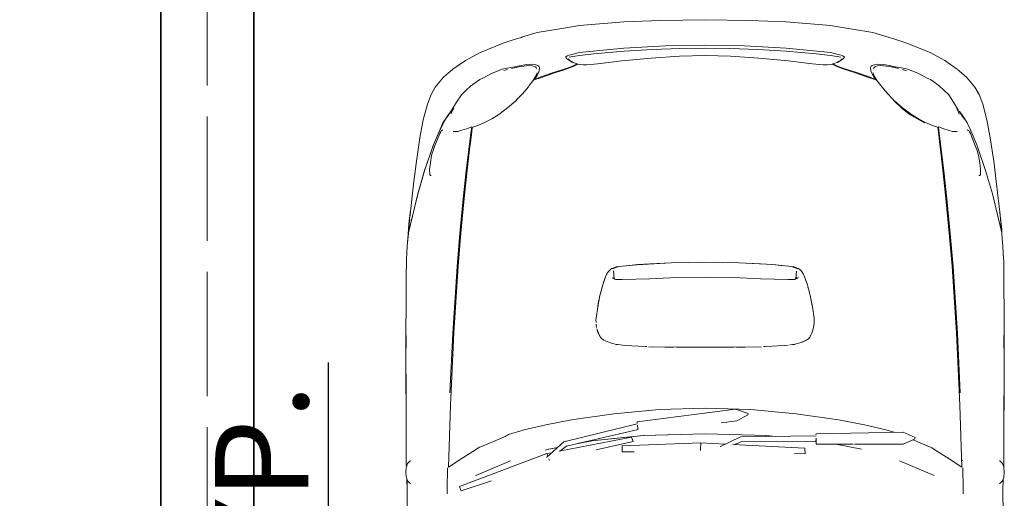
# Model space of a CAD drawing. Units: millimetres. Extents: x 595116 to 630915, y 909473 to 920225.
# Tile 117 of 134: x 629298 to 629393, y 919512 to 919558. Entities that reach past the tile are written whole.
import ezdxf

# ---------------------------------------------------------------- set-up
doc = ezdxf.new("R2010")
doc.units = ezdxf.units.MM
doc.linetypes.add('ACAD_ISO02W100', pattern=[15, 12, -3])
for name, color, linetype, lineweight in [('A-WALL', 1, 'Continuous', 35), ('C-PRKG-VEHI', 8, 'Continuous', 13), ('C-PROP-REF', 240, 'ACAD_ISO02W100', 13), ('Dimension', 3, 'Continuous', 18)]:
    doc.layers.add(name, color=color, linetype=linetype, lineweight=lineweight)
doc.styles.get("Standard").update_dxf_attribs({"font": 'arial.ttf'})
doc.dimstyles.new('ISO-25', dxfattribs={"dimtxt": 9, "dimasz": 6, "dimexe": 1.25, "dimexo": 0.625, "dimtad": 1, "dimlunit": 4, "dimtxsty": 'Standard', "dimcen": 2.5, "dimadec": 0, "dimazin": 0, "dimtfac": 1, "dimtmove": 0, "dimatfit": 3, "dimfxl": 1, "dimarcsym": 0})

# ---------------------------------------------------------------- blocks, each defined once
blk = doc.blocks.new('A$C7ADB3080')
for p, q in [((574.5, 1827.8), (485.6, 1817.6)), ((514, 1805.8), (622.7, 1832)), ((568.1, 1827.1), (601.7, 1831.6)), ((596.5, 1830), (587.6, 1828.8)), ((596.5, 1830), (598.5, 1830.3)), ((598.5, 1830.3), (629.8, 1833.4)), ((615.8, 1832.9), (601.7, 1831.6)), ((629.8, 1833.4), (615.8, 1832.9)), ((622.7, 1832), (625.4, 1832.6)), ((625.4, 1832.6), (622.7, 1832)), ((625.4, 1832.6), (627.4, 1832.8)), ((627.4, 1832.8), (625.4, 1832.6)), ((627.4, 1832.8), (629.3, 1833)), ((629.3, 1833), (627.4, 1832.8)), ((630.2, 1833.1), (628.2, 1832.8)), ((644.6, 1834.3), (629.8, 1833.4)), ((666, 1836.1), (630.2, 1833.1)), ((702.2, 1838.3), (666, 1836.1)), ((702.2, 1838.3), (704.4, 1838.4)), ((755.9, 1839.2), (704.4, 1838.4)), ((755.9, 1839.2), (789.1, 1839)), ((846.4, 1839.7), (789.1, 1839)), ((900.9, 1840.1), (846.4, 1839.7)), ((947, 1840.2), (900.9, 1840.1)), ((998.4, 1839.9), (923, 1839.2)), ((1014.5, 1840), (947, 1840.2)), ((998.4, 1839.9), (1014.5, 1840)), ((1066.5, 1839.8), (1014.5, 1840)), ((1117.5, 1839.5), (1066.5, 1839.8)), ((1120.4, 1839.3), (1070.3, 1839.6)), ((1164.2, 1839.3), (1117.5, 1839.5)), ((1120.4, 1839.3), (1164.2, 1839.1)), ((1164.2, 1839.1), (1164.1, 1839.1)), ((1186, 1839.2), (1164.2, 1839.3)), ((1211.9, 1839.1), (1164.4, 1839.2)), ((1256.2, 1839), (1211.9, 1839.1)), ((1295.5, 1839), (1256.2, 1839)), ((1284.8, 1825.7), (1285.6, 1828.2)), ((1285.6, 1828.2), (1292.6, 1835.1)), ((1292.6, 1835.1), (1302.3, 1838.5)), ((1295.5, 1839), (1302.9, 1838.7)), ((1302.3, 1838.5), (1304.4, 1839)), ((1304.4, 1839), (1317.7, 1840)), ((1331.1, 1839.1), (1317.7, 1840)), ((1331.1, 1839.1), (1333.2, 1838.5)), ((1342.9, 1835.1), (1333.2, 1838.5)), ((1336.7, 1837.3), (1371.1, 1836.1)), ((1349.8, 1828.2), (1342.9, 1835.1)), ((1350.6, 1825.4), (1349.8, 1828.2)), ((1371.1, 1836.1), (1377.3, 1836)), ((1377.3, 1836), (1430.5, 1836.5)), ((352.3, 1799.8), (300.5, 1789.8)), ((419.3, 1809.7), (352.3, 1799.8)), ((485.6, 1817.6), (419.3, 1809.7)), ((446.6, 1786.3), (514, 1805.8)), ((514, 1805.8), (446.6, 1786.3)), ((227, 1767.4), (205.8, 1755.4)), ((255.3, 1777.9), (227, 1767.4)), ((300.5, 1789.8), (255.3, 1777.9)), ((372.4, 1760.5), (446.6, 1786.3)), ((446.6, 1786.3), (372.4, 1760.5)), ((396.8, 1764.1), (391.9, 1762.5)), ((403.1, 1765.7), (396.8, 1764.1)), ((424.7, 1769.2), (403.1, 1765.7)), ((443.9, 1771.4), (424.7, 1769.2)), ((457.6, 1771.3), (443.9, 1771.4)), ((461, 1769.1), (457.6, 1771.3)), ((461.4, 1766.7), (461, 1769.1)), ((205.8, 1755.4), (177.4, 1731.2)), ((308.8, 1733), (327.4, 1741.3)), ((327.4, 1741.3), (308.8, 1733)), ((327.4, 1741.3), (372.4, 1760.5)), ((372.4, 1760.5), (327.4, 1741.3)), ((329.5, 1733), (330.6, 1736)), ((331.4, 1737.3), (330.6, 1736)), ((334.6, 1739.6), (331.4, 1737.3)), ((339.6, 1742.2), (334.6, 1739.6)), ((377.1, 1757.2), (339.6, 1742.2)), ((385.9, 1760.4), (377.1, 1757.2)), ((391.9, 1762.5), (385.9, 1760.4)), ((177.4, 1731.2), (154.5, 1704.8)), ((248.7, 1693.9), (272.8, 1708.2)), ((272.8, 1708.2), (248.7, 1693.9)), ((274.1, 1706.2), (268.7, 1703.4)), ((278, 1711.4), (275.4, 1709.5)), ((275.5, 1706.9), (283.4, 1709.5)), ((276.7, 1711.4), (284.8, 1717.1)), ((287.5, 1718), (278, 1711.4)), ((284.8, 1717.1), (296.4, 1724.9)), ((298.6, 1725.5), (287.5, 1718)), ((296.4, 1724.9), (308.8, 1733)), ((308.8, 1733), (296.4, 1724.9)), ((1124.1, 1711.4), (915.2, 1701.7)), ((917.2, 1704.7), (1089.1, 1712.9)), ((1303.7, 1717.2), (1124.1, 1711.4)), ((1279.1, 1680.6), (1303.7, 1717.2)), ((1284, 1719.6), (1282.1, 1716.5)), ((1304.9, 1720.3), (1365.2, 1721)), ((1365.2, 1721), (1380.7, 1721.1)), ((128.8, 1668.1), (153.9, 1704.5)), ((214.1, 1665.8), (228.3, 1679.7)), ((228.3, 1679.7), (214.1, 1665.8)), ((228.3, 1679.7), (248.7, 1693.9)), ((248.7, 1693.9), (228.3, 1679.7)), ((330.2, 1678.1), (326.2, 1665.2)), ((333.4, 1690.2), (330.2, 1678.1)), ((333.6, 1703.6), (333.4, 1690.2)), ((627.3, 1681.1), (536.8, 1672.6)), ((538.3, 1675.5), (628.6, 1684.1)), ((722.4, 1689.2), (627.3, 1681.1)), ((628.6, 1684.1), (723.6, 1692.3)), ((915.2, 1701.7), (722.4, 1689.2)), ((723.6, 1692.3), (917.2, 1704.7)), ((1257.7, 1647.2), (1279.1, 1680.6)), ((106.5, 1627.7), (128.8, 1668.1)), ((192.9, 1640.1), (202.7, 1653)), ((202.7, 1653), (192.9, 1640.1)), ((202.7, 1653), (214.1, 1665.8)), ((214.1, 1665.8), (202.7, 1653)), ((316.4, 1632.4), (321.9, 1649.9)), ((326.2, 1665.2), (320.7, 1650)), ((320.7, 1650), (340.1, 1652.4)), ((320.7, 1649.8), (320.7, 1650)), ((320.7, 1650), (321, 1650)), ((343.5, 1650.7), (321.3, 1648)), ((321.9, 1649.9), (322, 1650.2)), ((340.1, 1652.4), (392.9, 1659.3)), ((371.1, 1654.1), (343.5, 1650.7)), ((401.8, 1657.9), (371.1, 1654.1)), ((392.9, 1659.3), (455.7, 1666.7)), ((454.1, 1664), (401.8, 1657.9)), ((536.8, 1672.6), (454.1, 1664)), ((455.7, 1666.7), (538.2, 1675.4)), ((538.2, 1675.4), (538.2, 1675.4)), ((538.3, 1675.5), (538.3, 1675.5)), ((78.4, 1559.2), (106.5, 1627.7)), ((179.4, 1617.7), (183.6, 1626.9)), ((183.6, 1626.9), (179.4, 1617.7)), ((183.6, 1626.9), (192.9, 1640.1)), ((192.9, 1640.1), (183.6, 1626.9)), ((308, 1612.7), (316.4, 1632.4)), ((1224.6, 1577), (1244.4, 1624.1)), ((1244.4, 1624.1), (1245.8, 1627.5)), ((1245.8, 1627.5), (1247.6, 1630.5)), ((1247.6, 1630.5), (1257.7, 1647.2)), ((1285.5, 1538), (1327.9, 1638.1)), ((154.1, 1561.6), (166.6, 1592.6)), ((166.6, 1592.6), (154.1, 1561.6)), ((166.6, 1592.6), (179.4, 1617.7)), ((179.4, 1617.7), (166.6, 1592.6)), ((284.8, 1567.7), (299.6, 1592.1)), ((285.2, 1572), (297.6, 1592.1)), ((297.6, 1592.1), (308, 1612.7)), ((299.6, 1592.1), (308.6, 1609.9)), ((265.7, 1546.2), (285.2, 1572)), ((284.8, 1567.7), (268.5, 1546.6)), ((284.8, 1567.7), (284.7, 1567.6)), ((1201.9, 1547.7), (1217.9, 1583.1)), ((1223, 1580.9), (1217.9, 1583.1)), ((1236.7, 1548.1), (1223, 1580.9)), ((70.3, 1532.9), (78.4, 1559.2)), ((147.2, 1525.2), (150.6, 1548.3)), ((150.6, 1548.3), (147.2, 1525.2)), ((150.6, 1548.3), (154.1, 1561.6)), ((154.1, 1561.6), (150.6, 1548.3)), ((158.2, 1557.5), (154.9, 1546.4)), ((245.7, 1523), (265.7, 1546.2)), ((268.5, 1546.6), (247.9, 1525.1)), ((1207.6, 1296.6), (1201.9, 1547.7)), ((1236.9, 1407.5), (1236.7, 1548.1)), ((1285.3, 1537.6), (1285.5, 1538)), ((62.1, 1506.7), (66.6, 1521)), ((66.6, 1521), (70.3, 1532.9)), ((140.7, 1492.2), (144.6, 1512.1)), ((144.6, 1512.1), (140.7, 1492.2)), ((145.9, 1508), (143.4, 1483.5)), ((144.6, 1512.1), (147.2, 1525.2)), ((147.2, 1525.2), (144.6, 1512.1)), ((150.3, 1526.6), (145.9, 1508)), ((152.2, 1535), (150.3, 1526.6)), ((237.6, 1515.3), (225.8, 1504.4)), ((247.9, 1525.1), (237.6, 1515.3)), ((1195.1, 1498.2), (1202.5, 1522)), ((61.6, 1504.8), (48.4, 1460.7)), ((61.6, 1504.8), (62.1, 1506.7)), ((139.4, 1475.5), (140.7, 1492.2)), ((140.7, 1492.2), (139.4, 1475.5)), ((143.4, 1483.5), (144.5, 1474.1)), ((201, 1483.7), (187.2, 1473)), ((204.5, 1486.1), (201, 1483.7)), ((217.4, 1496.7), (204.5, 1486.1)), ((225.8, 1504.4), (217.4, 1496.7)), ((1180.7, 1436.4), (1195.1, 1498.2)), ((48.4, 1460.7), (38.4, 1401.7)), ((140.1, 1468.1), (139.4, 1475.5)), ((139.4, 1475.5), (140.1, 1468.1)), ((143.2, 1458.9), (140.1, 1468.1)), ((140.1, 1468.1), (143.2, 1458.9)), ((145, 1456.1), (143.2, 1458.9)), ((143.2, 1458.9), (145, 1456.1)), ((144.5, 1474.1), (146.2, 1469.1)), ((148.9, 1454.2), (145, 1456.1)), ((145, 1456.1), (148.9, 1454.2)), ((146.5, 1468.2), (149.1, 1464)), ((160, 1454.9), (148.9, 1454.2)), ((148.9, 1454.2), (160, 1454.9)), ((149.1, 1464), (151.7, 1462.6)), ((172.4, 1461.2), (160, 1454.9)), ((160, 1454.9), (172.4, 1461.2)), ((162.7, 1410.7), (176.1, 1450.1)), ((164.5, 1461.2), (172.2, 1463.8)), ((178.9, 1450.6), (164.5, 1410.7)), ((172, 1462.5), (184.5, 1470.4)), ((172.2, 1463.8), (181.7, 1469.2)), ((183.7, 1468.4), (172.4, 1461.2)), ((172.4, 1461.2), (183.7, 1468.4)), ((174.2, 1464.8), (173.9, 1464.7)), ((174.8, 1465.1), (174.2, 1464.8)), ((176.1, 1450.1), (183.7, 1468.4)), ((184.7, 1470.2), (178.9, 1450.6)), ((181.7, 1469.2), (186.7, 1472.5)), ((183.5, 1468), (184.1, 1468.1)), ((183.7, 1468.4), (184.5, 1470.4)), ((184, 1469.2), (184.5, 1469.5)), ((184.1, 1469.5), (184.6, 1469.7)), ((184.5, 1470.4), (185.1, 1470.6)), ((187.2, 1473), (184.7, 1470.2)), ((1166.8, 1361.5), (1180.7, 1436.4)), ((1237, 1353.9), (1251.4, 1427.7)), ((27.8, 1338.5), (38.4, 1401.7)), ((154.5, 1385.6), (162.7, 1410.7)), ((164.5, 1410.7), (156.5, 1386)), ((1237.1, 1297.2), (1236.9, 1403.7)), ((112.3, 1364.4), (113.8, 1369.4)), ((113.8, 1369.4), (112.3, 1364.4)), ((113.8, 1369.4), (115.5, 1374.4)), ((115.5, 1374.4), (113.8, 1369.4)), ((115.5, 1374.4), (118, 1378)), ((118, 1378), (115.5, 1374.4)), ((118.7, 1368.1), (117, 1357.9)), ((118, 1378), (119.5, 1378.4)), ((119.5, 1378.4), (118, 1378)), ((119.5, 1378.4), (123.8, 1375.2)), ((123.8, 1375.2), (119.5, 1378.4)), ((123.7, 1371.6), (127.9, 1368.1)), ((123.8, 1375.2), (127.7, 1369.2)), ((127.7, 1369.2), (123.8, 1375.2)), ((127.7, 1369.2), (133.5, 1360.1)), ((133.5, 1360.1), (127.7, 1369.2)), ((127.9, 1368.1), (131.7, 1361.7)), ((145.3, 1358.5), (150.2, 1371.5)), ((151.3, 1369.4), (145.6, 1354.8)), ((150.2, 1371.5), (154.5, 1385.6)), ((156.5, 1386), (151.3, 1369.4)), ((27.8, 1338.5), (17, 1210.7)), ((93.5, 1210.7), (105.3, 1338.7)), ((105.3, 1338.7), (93.5, 1210.7)), ((105.3, 1338.7), (112.3, 1364.4)), ((112.3, 1364.4), (105.3, 1338.7)), ((114.6, 1338.6), (109.6, 1297.4)), ((117, 1357.9), (114.6, 1338.6)), ((131.7, 1361.7), (134.5, 1357.5)), ((133.5, 1360.1), (137.9, 1348.2)), ((137.9, 1348.2), (133.5, 1360.1)), ((137.9, 1348.2), (138.7, 1345.5)), ((138.7, 1345.5), (137.9, 1348.2)), ((138.7, 1345.5), (145.3, 1358.5)), ((140.3, 1345.5), (138.7, 1345.5)), ((145.6, 1354.8), (139.2, 1343.6)), ((139.2, 1343.6), (140.6, 1338.5)), ((140.1, 1345.5), (140.2, 1345.3)), ((140.6, 1338.5), (141.3, 1328.4)), ((1149.4, 1239.2), (1166.8, 1361.5)), ((141, 1317.4), (140.1, 1305.8)), ((141.3, 1328.4), (141, 1317.4)), ((109.6, 1297.4), (102.1, 1210)), ((138.4, 1286.6), (135.7, 1262.5)), ((140.1, 1305.8), (138.4, 1286.6)), ((807.2, 1279.5), (776.6, 1271.5)), ((840.1, 1286.2), (807.2, 1279.5)), ((816.8, 1281.5), (831.5, 1284.8)), ((831.5, 1284.8), (838.3, 1285.8)), ((873.1, 1290.9), (840.1, 1286.2)), ((888.8, 1291.1), (873.1, 1290.9)), ((873.2, 1290.9), (876.6, 1291.3)), ((876.6, 1291.3), (884.9, 1291)), ((903.4, 1288.7), (888.8, 1291.1)), ((890.4, 1290.8), (894.1, 1290.7)), ((894.1, 1290.7), (899.9, 1289.3)), ((916.5, 1284.3), (903.4, 1288.7)), ((906.8, 1287.6), (908, 1287.3)), ((908, 1287.3), (916.4, 1284.4)), ((916.4, 1284.4), (923.9, 1280.5)), ((927.7, 1278.5), (916.5, 1284.3)), ((923.9, 1280.5), (924.7, 1280.1)), ((1207.6, 1296.6), (1209.6, 1296.4)), ((1215.8, 1078.8), (1213.2, 1296.7)), ((1227.6, 1296), (1219.5, 1296.9)), ((1222.6, 1296.6), (1237.1, 1297.2)), ((1226.3, 1296.1), (1226.4, 1296.8)), ((1230.4, 1295.7), (1227.6, 1296)), ((1229.7, 1083), (1230.4, 1295.7)), ((135.7, 1262.5), (129.8, 1216.2)), ((737.5, 1254.5), (732.6, 1249.6)), ((743.3, 1258.9), (737.5, 1254.5)), ((750.3, 1262.4), (743.3, 1258.9)), ((744.9, 1259.7), (745.5, 1260.1)), ((745.5, 1260.1), (746.8, 1260.6)), ((776.6, 1271.5), (750.3, 1262.4)), ((755.5, 1264.2), (760.9, 1266.4)), ((760.9, 1266.4), (769.9, 1269.2)), ((783.2, 1273.2), (791.1, 1275.6)), ((791.1, 1275.6), (800.2, 1277.7)), ((931.6, 1275.4), (927.7, 1278.5)), ((928.5, 1277.9), (929.6, 1277.2)), ((929.6, 1277.2), (930.1, 1276.6)), ((934.3, 1272), (931.6, 1275.4)), ((936.3, 1268.2), (934.3, 1272)), ((935.3, 1270), (936.3, 1268.7)), ((936.3, 1268.7), (941.9, 1256.9)), ((938.5, 1264), (936.3, 1268.2)), ((944.5, 1249.5), (938.5, 1264)), ((941.9, 1256.9), (943, 1253.2)), ((1248.6, 1264.5), (1238.1, 1056.7)), ((1264.7, 1265), (1248.6, 1264.5)), ((1263.8, 1234.3), (1264.7, 1265)), ((724, 1225.9), (718.5, 1171.5)), ((730.7, 1243.7), (724, 1225.9)), ((724.5, 1227.4), (725.2, 1233.3)), ((725.2, 1233.3), (729.7, 1243.8)), ((732.6, 1249.6), (728.6, 1244.4)), ((728.6, 1244.4), (730.5, 1243.3)), ((733.1, 1250.3), (733, 1250.1)), ((733.3, 1250.3), (733.1, 1250.3)), ((758.8, 1237.8), (737.6, 1240.5)), ((755.9, 1240.9), (761.1, 1235.4)), ((755.9, 1240.9), (755.9, 1240.9)), ((756.6, 1246), (761.8, 1233.7)), ((756.8, 1244), (759.3, 1239.6)), ((756.8, 1244), (756.8, 1244)), ((761.5, 1215.3), (761.8, 1234)), ((948.4, 1236.1), (944.5, 1249.5)), ((950.5, 1221.1), (948.4, 1236.1)), ((948.6, 1234.4), (949, 1233.2)), ((949, 1233.2), (949.6, 1227.7)), ((1137.2, 1107.4), (1149.4, 1239.2)), ((17, 1210.7), (13, 1104.1)), ((86.9, 1090.2), (93.5, 1210.7)), ((93.5, 1210.7), (86.9, 1090.2)), ((102.1, 1210), (97.3, 1128.3)), ((129.8, 1216.2), (121.7, 1131.5)), ((718.5, 1171.7), (721.7, 1202.7)), ((721.7, 1202.7), (721.7, 1203)), ((761.5, 1215.3), (759.2, 1135.8)), ((950.8, 1216.3), (951.9, 1206.7)), ((951.9, 1206.7), (954.9, 1149.6)), ((718.5, 1171.5), (712.9, 1074.6)), ((716.1, 1136.1), (718.5, 1171.7)), ((1212, 1154.3), (1214.6, 1179.7)), ((1214.6, 1179.7), (1212.1, 1154.5)), ((954.9, 1149.6), (955.1, 1144.6)), ((956.9, 1058.9), (955.4, 1139.5)), ((1212.1, 1154.5), (1207, 976.2)), ((1207, 976.2), (1212, 1154.3)), ((97.3, 1128.3), (94.3, 1048.9)), ((121.7, 1131.5), (116.6, 1049.9)), ((712.8, 1074.5), (716.1, 1136.1)), ((759.2, 1135.8), (755.9, 1058.6)), ((955.6, 1128.3), (956.8, 1091.9)), ((13, 1104.1), (11.7, 976.2)), ((84.7, 976.2), (86.9, 1090.2)), ((86.9, 1090.2), (84.7, 976.2)), ((956.8, 1091.9), (956.8, 1066.5)), ((1132.6, 976.2), (1137.2, 1107.4)), ((1135.7, 1064.3), (1148.4, 1101)), ((1152, 1099.3), (1148.4, 1101)), ((1169.8, 1068.2), (1152, 1099.3)), ((1238.3, 1061.1), (1229.7, 1083)), ((712.9, 1074.6), (711.4, 976.2)), ((711.4, 976.2), (712.8, 1074.5)), ((755.9, 1058.6), (754.2, 976.2)), ((957.1, 976.2), (956.9, 1058.9)), ((1172.6, 779.7), (1135.7, 1063.8)), ((1174.9, 1022.3), (1169.8, 1068.2)), ((1243.9, 1020.7), (1215.8, 1078.8)), ((94.3, 1048.9), (93.3, 976.2)), ((116.6, 1049.9), (114.8, 976.2)), ((1237, 1034.9), (1233.4, 963.6)), ((1243.9, 1020.7), (1244.3, 1020.7)), ((11.7, 976.2), (13, 848.2)), ((86.9, 862.1), (84.7, 976.2)), ((84.7, 976.2), (86.9, 862.1)), ((93.3, 976.2), (94.3, 903.4)), ((114.8, 976.2), (116.6, 902.5)), ((711.4, 976.2), (712.9, 877.9)), ((712.8, 877.9), (711.4, 976.2)), ((754.2, 976.2), (755.9, 893.8)), ((956.9, 893.5), (957.1, 976.2)), ((1137.2, 845), (1132.6, 976.2)), ((1212, 798.1), (1207, 976.2)), ((1207, 976.2), (1212.1, 797.9)), ((1233.4, 963.6), (1242, 736.5)), ((1251.9, 963.2), (1233.4, 963.6)), ((1254.9, 963.3), (1251.9, 963.2)), ((94.3, 903.4), (97.3, 824.1)), ((116.6, 902.5), (121.7, 820.9)), ((755.9, 893.8), (759.2, 816.6)), ((955.4, 812.9), (956.9, 893.5)), ((956.8, 885.8), (956.8, 860.5)), ((93.5, 741.7), (86.9, 862.1)), ((86.9, 862.1), (93.5, 741.7)), ((716.1, 816.3), (712.8, 877.9)), ((712.9, 877.9), (718.6, 779.9)), ((956.8, 860.5), (955.6, 824.1)), ((13, 848.2), (17, 741.7)), ((1149.4, 713.2), (1137.2, 845)), ((97.3, 824.1), (102.1, 742.4)), ((121.7, 820.9), (129.8, 736.1)), ((718.5, 780.7), (716.1, 816.3)), ((759.2, 816.6), (761.5, 737.1)), ((954.9, 802.8), (951.9, 745.7)), ((955.1, 807.8), (954.9, 802.8)), ((1227, 649.4), (1212, 798.1)), ((1212.1, 797.9), (1222.5, 694.4)), ((721.6, 749.8), (718.5, 780.7)), ((718.6, 779.9), (724, 726.5)), ((1172.6, 779.7), (1175.9, 779.9)), ((1230.5, 568.5), (1178, 780.4)), ((1193.1, 782.3), (1182.2, 781)), ((1193.9, 782.6), (1193.1, 782.3)), ((1242.6, 576.1), (1194.9, 782.6)), ((1228.9, 768.7), (1217.2, 764.2)), ((1253.7, 662.2), (1228.9, 768.7)), ((1259.1, 737.2), (1258.7, 771.2)), ((17, 741.7), (27.8, 613.9)), ((105.3, 613.6), (93.5, 741.7)), ((93.5, 741.7), (105.3, 613.6)), ((102.1, 742.4), (109.6, 654.9)), ((951.9, 745.7), (950.5, 731.3)), ((1217.2, 764.2), (1257.5, 555)), ((129.8, 736.1), (135.7, 689.9)), ((724, 726.5), (730.7, 708.6)), ((725.2, 719.1), (724.5, 725)), ((729.7, 708.6), (725.2, 719.1)), ((758.4, 714.2), (736.5, 711.7)), ((755.9, 711.5), (761, 717)), ((756.8, 708.4), (761.8, 718.7)), ((761.5, 737.1), (761.8, 718.7)), ((944.5, 702.9), (948.4, 716.3)), ((948.4, 716.3), (950.5, 731.3)), ((949.6, 724.7), (949, 719.2)), ((1166.8, 590.9), (1149.4, 713.2)), ((1242, 736.5), (1258.1, 737)), ((1259.1, 737.2), (1258.1, 737)), ((135.7, 689.9), (138.4, 665.8)), ((730.5, 709), (728.6, 708)), ((728.6, 708), (732.6, 702.8)), ((732.6, 702.8), (737.5, 697.9)), ((733, 702.3), (733.1, 702.1)), ((733.1, 702.1), (733.3, 702.1)), ((737.5, 697.9), (743.3, 693.5)), ((743.3, 693.5), (750.3, 690)), ((745.5, 692.3), (744.9, 692.7)), ((746.8, 691.7), (745.5, 692.3)), ((750.3, 690), (776.6, 680.9)), ((760.9, 685.9), (755.5, 688.2)), ((769.9, 683.2), (760.9, 685.9)), ((931.6, 677), (936.3, 684.2)), ((936.3, 684.2), (938.5, 688.3)), ((938.5, 688.3), (944.5, 702.9)), ((109.6, 654.9), (114.6, 613.7)), ((138.4, 665.8), (140.1, 646.5)), ((776.6, 680.9), (807.2, 672.8)), ((791.1, 676.8), (783.2, 679.2)), ((800.2, 674.7), (791.1, 676.8)), ((807.2, 672.8), (840.1, 666.2)), ((831.5, 667.6), (816.8, 670.9)), ((838.3, 666.6), (831.5, 667.6)), ((840.1, 666.2), (873.1, 661.5)), ((876.6, 661), (873.2, 661.5)), ((885.2, 661.3), (876.6, 661)), ((894.1, 661.6), (890.2, 661.5)), ((900.1, 663.2), (894.1, 661.6)), ((903.4, 663.7), (916.5, 668.1)), ((908, 665.1), (906.7, 664.8)), ((916.4, 668), (908, 665.1)), ((923.9, 671.8), (916.4, 668)), ((916.5, 668.1), (927.7, 673.9)), ((925.2, 672.6), (923.9, 671.8)), ((927.7, 673.9), (931.6, 677)), ((140.1, 646.5), (141, 635)), ((141, 635), (141.3, 624)), ((1227, 649.8), (1234.6, 610.6)), ((1234.5, 611.2), (1227, 649.4)), ((38.4, 550.7), (27.8, 613.9)), ((112.3, 588), (105.3, 613.6)), ((105.3, 613.6), (112.3, 588)), ((114.6, 613.7), (117, 594.4)), ((137.9, 604.2), (133.5, 592.2)), ((133.5, 592.2), (137.9, 604.2)), ((138.7, 606.9), (137.9, 604.2)), ((137.9, 604.2), (138.7, 606.9)), ((145.3, 593.9), (138.7, 606.9)), ((138.7, 606.9), (140.3, 606.9)), ((140.6, 613.9), (139.2, 608.8)), ((139.2, 608.8), (145.6, 597.6)), ((140.2, 607), (140.2, 606.9)), ((141.3, 624), (140.6, 613.9)), ((145.6, 597.6), (151.3, 583)), ((113.8, 583), (112.3, 588)), ((112.3, 588), (113.8, 583)), ((115.5, 577.9), (113.8, 583)), ((113.8, 583), (115.5, 577.9)), ((118, 574.3), (115.5, 577.9)), ((115.5, 577.9), (118, 574.3)), ((117, 594.4), (118.7, 584.2)), ((119.5, 573.9), (118, 574.3)), ((118, 574.3), (119.5, 573.9)), ((123.8, 577.2), (119.5, 573.9)), ((119.5, 573.9), (123.8, 577.2)), ((127.9, 584.3), (123.7, 580.8)), ((127.7, 583.2), (123.8, 577.2)), ((123.8, 577.2), (127.7, 583.2)), ((133.5, 592.2), (127.7, 583.2)), ((127.7, 583.2), (133.5, 592.2)), ((131.7, 590.6), (127.9, 584.3)), ((134.5, 594.9), (131.7, 590.6)), ((150.2, 580.9), (145.3, 593.9)), ((154.5, 566.8), (150.2, 580.9)), ((151.3, 583), (156.5, 566.4)), ((1180.7, 516), (1166.8, 590.9)), ((1257.1, 557), (1242.6, 576.1)), ((38.4, 550.7), (48.4, 491.6)), ((162.7, 541.6), (154.5, 566.8)), ((156.5, 566.4), (164.5, 541.7)), ((176.1, 502.3), (162.7, 541.6)), ((164.5, 541.7), (178.9, 501.8)), ((1274.5, 519), (1230.5, 568.5)), ((1251.4, 524.6), (1246.3, 550.8)), ((1246.3, 550.8), (1251.4, 524.7)), ((1195.1, 454.2), (1180.7, 516)), ((1251.4, 524.7), (1251.4, 524.6)), ((1254.1, 515.9), (1251.4, 524.6)), ((1261.6, 533.5), (1264.2, 519.8)), ((1271.7, 522.2), (1264.2, 519.8)), ((1264.2, 519.8), (1359.7, 267.1)), ((1274.5, 519), (1275, 519.1)), ((1282.4, 525.7), (1279.7, 524.8)), ((1284.5, 526.7), (1282.4, 525.7)), ((1284.5, 526.7), (1282.4, 525.7)), ((61.8, 446.6), (48.4, 491.6)), ((140.1, 484.3), (139.4, 476.9)), ((139.4, 476.9), (140.1, 484.3)), ((143.2, 493.4), (140.1, 484.3)), ((140.1, 484.3), (143.2, 493.4)), ((145, 496.2), (143.2, 493.4)), ((143.2, 493.4), (145, 496.2)), ((148.9, 498.2), (145, 496.2)), ((145, 496.2), (148.9, 498.2)), ((149.1, 488.4), (146.5, 484.2)), ((160, 497.5), (148.9, 498.2)), ((148.9, 498.2), (160, 497.5)), ((151.9, 489.8), (149.1, 488.4)), ((172.4, 491.2), (160, 497.5)), ((160, 497.5), (172.4, 491.2)), ((172.2, 488.6), (164.5, 491.2)), ((181.7, 483.1), (172.2, 488.6)), ((183.7, 484), (172.4, 491.2)), ((172.4, 491.2), (183.7, 484)), ((183.7, 484), (176.1, 502.3)), ((178.9, 501.8), (184.7, 482.1)), ((184.5, 482), (183.7, 484)), ((139.4, 476.9), (140.7, 460.2)), ((140.7, 460.2), (139.4, 476.9)), ((140.7, 460.2), (144.6, 440.3)), ((144.6, 440.3), (140.7, 460.2)), ((144.5, 478.2), (143.4, 468.8)), ((143.4, 468.8), (145.9, 444.4)), ((146.2, 483.2), (144.5, 478.2)), ((186.8, 479.9), (181.7, 483.1)), ((185.1, 481.8), (184.5, 482)), ((184.7, 482.1), (187.2, 479.3)), ((187.2, 479.3), (201, 468.7)), ((201, 468.7), (204.5, 466.3)), ((204.5, 466.3), (217.4, 455.7)), ((217.4, 455.7), (225.8, 447.9)), ((62.1, 445.7), (61.6, 447.5)), ((66.6, 431.3), (62.1, 445.7)), ((70.3, 419.5), (66.6, 431.3)), ((144.6, 440.3), (147.2, 427.2)), ((147.2, 427.2), (144.6, 440.3)), ((145.9, 444.4), (150.3, 425.8)), ((147.2, 427.2), (150.6, 404)), ((150.6, 404), (147.2, 427.2)), ((225.8, 447.9), (237.6, 437)), ((237.6, 437), (247.9, 427.3)), ((265.7, 406.2), (245.5, 429.5)), ((1209.1, 409.1), (1195.1, 454.2)), ((78.4, 393.2), (70.3, 419.5)), ((150.3, 425.8), (152.2, 417.4)), ((150.6, 404), (154.1, 390.7)), ((154.1, 390.7), (150.6, 404)), ((154.9, 405.9), (158.1, 394.9)), ((285.2, 380.4), (265.7, 406.2)), ((1211.1, 405.7), (1209.1, 409.1)), ((1213.2, 402.1), (1211.1, 405.7)), ((1214.7, 399.2), (1213.2, 402.1)), ((1215.6, 397), (1214.7, 399.2)), ((1285.5, 414.4), (1285.3, 414.8)), ((1327.9, 314.3), (1285.5, 414.4)), ((106.5, 324.6), (78.4, 393.2)), ((154.1, 390.7), (166.6, 359.8)), ((166.6, 359.8), (154.1, 390.7)), ((297.6, 360.3), (285.2, 380.4)), ((1244.4, 328.3), (1215.6, 397)), ((166.6, 359.8), (179.4, 334.6)), ((179.4, 334.6), (166.6, 359.8)), ((308, 339.7), (297.6, 360.3)), ((1372.2, 272.1), (1342.5, 359.1)), ((128.8, 284.3), (106.5, 324.6)), ((179.4, 334.6), (183.6, 325.4)), ((183.6, 325.4), (179.4, 334.6)), ((183.6, 325.4), (192.9, 312.3)), ((192.9, 312.3), (183.6, 325.4)), ((316.4, 319.9), (308, 339.7)), ((321.9, 302.5), (316.4, 319.9)), ((1245.8, 324.9), (1244.4, 328.3)), ((1247.6, 321.8), (1245.8, 324.9)), ((1257.7, 305.2), (1247.6, 321.8)), ((1328, 314.1), (1327.9, 314.3)), ((153.9, 247.9), (128.8, 284.3)), ((192.9, 312.3), (202.7, 299.4)), ((202.7, 299.4), (192.9, 312.3)), ((202.7, 299.4), (214.1, 286.6)), ((214.1, 286.6), (202.7, 299.4)), ((214.1, 286.6), (228.3, 272.7)), ((228.3, 272.7), (214.1, 286.6)), ((320.7, 302.4), (320.7, 302.6)), ((340.1, 300), (320.7, 302.4)), ((320.7, 302.4), (326.2, 287.1)), ((321, 302.4), (320.7, 302.4)), ((322, 302.2), (321.9, 302.5)), ((323.2, 304.2), (323.4, 304.1)), ((323.9, 302.5), (323.4, 304.1)), ((323.4, 304.1), (343.5, 301.6)), ((324.1, 301.9), (323.9, 302.5)), ((324.8, 302.3), (324, 302.3)), ((326.2, 287.1), (330.2, 274.3)), ((326.6, 303.7), (326.9, 302)), ((328.2, 302.2), (326.9, 302.3)), ((328.2, 303.5), (328.2, 302.2)), ((392.9, 293.1), (340.1, 300)), ((343.5, 301.6), (371.1, 298.2)), ((371.1, 298.2), (401.8, 294.5)), ((455.7, 285.7), (392.9, 293.1)), ((401.8, 294.5), (454.1, 288.4)), ((454.1, 288.4), (536.8, 279.7)), ((538.2, 276.9), (455.7, 285.7)), ((1279.1, 271.8), (1257.7, 305.2)), ((228.3, 272.7), (248.7, 258.4)), ((248.7, 258.4), (228.3, 272.7)), ((248.7, 258.4), (272.8, 244.2)), ((272.8, 244.2), (248.7, 258.4)), ((330.2, 274.3), (333.4, 262.2)), ((333.4, 262.2), (333.6, 248.8)), ((536.8, 279.7), (627.3, 271.2)), ((538.2, 276.9), (538.2, 276.9)), ((628.6, 268.2), (538.3, 276.9)), ((538.3, 276.9), (538.3, 276.9)), ((627.3, 271.2), (722.4, 263.1)), ((723.6, 260.1), (628.6, 268.2)), ((722.4, 263.1), (915.2, 250.7)), ((917.2, 247.7), (723.6, 260.1)), ((1303.7, 235.1), (1279.1, 271.8)), ((1359.7, 267.1), (1371.5, 271.7)), ((1372.2, 272.1), (1371.5, 271.7)), ((156.5, 245), (153.9, 247.9)), ((154, 247.9), (177.4, 221.2)), ((273.8, 245.9), (266.3, 250.4)), ((268.3, 249.3), (274.1, 246.2)), ((272.8, 244.2), (273.8, 245.9)), ((274.3, 244.9), (272.8, 244.2)), ((272.8, 244.2), (276.7, 241)), ((276.7, 241), (272.8, 244.2)), ((274.1, 246.2), (277, 244.9)), ((275.5, 245.4), (274.2, 244.9)), ((275.4, 242.9), (274.2, 244.9)), ((275.4, 242.9), (278, 241)), ((283, 243), (275.5, 245.4)), ((276.7, 241), (284.8, 235.3)), ((284.8, 235.3), (276.7, 241)), ((298.6, 226.9), (278, 241)), ((278, 241), (287.5, 234.4)), ((284.8, 235.3), (296.4, 227.4)), ((296.4, 227.4), (284.8, 235.3)), ((287.5, 234.4), (298.6, 226.9)), ((296.4, 227.4), (308.8, 219.4)), ((308.8, 219.4), (296.4, 227.4)), ((915.2, 250.7), (1124.1, 241)), ((1089.1, 239.4), (917.2, 247.7)), ((1089.1, 239.4), (1089.1, 239.4)), ((1124.1, 241), (1303.7, 235.1)), ((1365.2, 231.3), (1304.9, 232.1)), ((1380.7, 231.3), (1365.2, 231.3)), ((177.4, 221.2), (205.8, 197)), ((327.9, 211.4), (298.6, 226.9)), ((298.6, 226.9), (310.9, 219)), ((308.8, 219.4), (327.4, 211.1)), ((327.4, 211.1), (308.8, 219.4)), ((310.9, 219), (327.9, 211.4)), ((327.4, 211.1), (372.4, 191.8)), ((372.4, 191.8), (327.4, 211.1)), ((327.9, 211.4), (374.7, 191.5)), ((330.6, 216.3), (329.5, 219.4)), ((330.6, 216.3), (331.4, 215.1)), ((331.4, 215.1), (334.6, 212.8)), ((334.6, 212.8), (339.6, 210.2)), ((339.6, 210.2), (377.1, 195.2)), ((205.8, 197), (227, 185)), ((227, 185), (255.3, 174.5)), ((255.3, 174.5), (300.5, 162.6)), ((372.4, 191.8), (446.6, 166.1)), ((446.6, 166.1), (372.4, 191.8)), ((374.7, 191.5), (447.7, 166.2)), ((377.1, 195.2), (385.9, 191.9)), ((385.9, 191.9), (391.9, 189.9)), ((391.9, 189.9), (396.8, 188.3)), ((396.8, 188.3), (403.1, 186.6)), ((403.1, 186.6), (424.7, 183.2)), ((424.7, 183.2), (443.9, 181)), ((443.9, 181), (457.6, 181.1)), ((457.6, 181.1), (461, 183.3)), ((461, 183.3), (461.4, 185.7)), ((300.5, 162.6), (352.3, 152.6)), ((352.3, 152.6), (419.3, 142.7)), ((419.3, 142.7), (485.6, 134.8)), ((446.6, 166.1), (514, 146.6)), ((514, 146.6), (446.6, 166.1)), ((447.7, 166.2), (515, 146.7)), ((514, 146.6), (622.7, 120.4)), ((622.7, 120.4), (514, 146.6)), ((515, 146.7), (625.4, 120.1)), ((515, 146.7), (515, 146.7)), ((485.6, 134.8), (582.2, 123.9)), ((529.7, 129.8), (574.5, 124.6)), ((568.1, 125.2), (562.5, 126)), ((601.7, 120.8), (568.1, 125.2)), ((587.6, 123.6), (596.5, 122.4)), ((598.5, 122.1), (596.5, 122.4)), ((598.5, 122.1), (627.4, 119.5)), ((601.7, 120.8), (615.8, 119.5)), ((615.8, 119.5), (629.8, 119)), ((622.7, 120.4), (625.4, 119.8)), ((625.4, 119.8), (622.7, 120.4)), ((625.4, 120.2), (625.4, 120.1)), ((625.4, 120.1), (628.2, 119.5)), ((625.4, 119.8), (627.4, 119.5)), ((627.4, 119.5), (625.4, 119.8)), ((627.4, 119.5), (629, 119.4)), ((629, 119.4), (627.4, 119.5)), ((628.2, 119.5), (664.3, 116.4)), ((628.2, 119.5), (628.3, 119.5)), ((628.2, 119.5), (630.2, 119.3)), ((629.8, 119), (644.6, 118.1)), ((630.2, 119.3), (666, 116.3)), ((664.3, 116.4), (666, 116.3)), ((666, 116.3), (702.2, 114)), ((704.4, 113.9), (702.2, 114)), ((704.4, 113.9), (755.9, 113.2)), ((1285.6, 124.1), (1284.8, 126.6)), ((1292.6, 117.3), (1285.6, 124.1)), ((1302.3, 113.9), (1292.6, 117.3)), ((1304.4, 113.3), (1302.3, 113.9)), ((1333.2, 113.9), (1331.1, 113.3)), ((1333.2, 113.9), (1342.9, 117.3)), ((1370.4, 116.3), (1336.6, 115.1)), ((1339.7, 116.2), (1377.3, 116.3)), ((1342.9, 117.3), (1349.8, 124.1)), ((1349.8, 124.1), (1350.6, 126.9)), ((1430.5, 115.9), (1377.3, 116.3)), ((789.1, 113.4), (755.9, 113.2)), ((789.1, 113.4), (846.4, 112.7)), ((846.4, 112.7), (900.9, 112.3)), ((900.9, 112.3), (947, 112.2)), ((923, 113.1), (998.4, 112.5)), ((923, 113.1), (923, 113.1)), ((947, 112.2), (1014.5, 112.4)), ((998.4, 112.5), (1070.6, 112.8)), ((1014.5, 112.4), (998.4, 112.5)), ((1014.5, 112.4), (1066.5, 112.6)), ((1066.5, 112.6), (1117.5, 112.8)), ((1120.4, 113.1), (1070.6, 112.8)), ((1117.5, 112.8), (1164.2, 113.1)), ((1120.3, 113.1), (1120.4, 113.1)), ((1164.2, 113.1), (1186, 113.2)), ((1164.4, 113.2), (1211.9, 113.3)), ((1211.9, 113.3), (1256.2, 113.3)), ((1256.2, 113.3), (1295.5, 113.4)), ((1302.9, 113.7), (1295.5, 113.4)), ((1317.7, 112.4), (1304.4, 113.3)), ((1317.7, 112.4), (1331.1, 113.3))]:
    blk.add_line(p, q)
blk = doc.blocks.new('*D128')
at = {"layer": 'Defpoints', "color": 0, "transparency": 16777216}
for p in [(629311.541, 920089.428), (629282.395, 919141.928), (629311.541, 919141.928)]:
    blk.add_point(p, dxfattribs=at)
at = {"layer": 'Dimension', "color": 0, "lineweight": -2, "transparency": 16777216}
for p, q in [((629310.916, 920089.428), (629281.145, 920089.428)), ((629282.395, 920083.428), (629282.395, 919147.928)), ((629310.916, 919141.928), (629281.145, 919141.928))]:
    blk.add_line(p, q, dxfattribs=at)
at = {"layer": 'Dimension', "color": 0, "transparency": 16777216}
for points in [[(629281.395, 920083.428), (629283.395, 920083.428), (629282.395, 920089.428)], [(629281.395, 919147.928), (629283.395, 919147.928), (629282.395, 919141.928)]]:
    blk.add_solid(points, dxfattribs=at)
at = {"layer": 'Dimension', "color": 0, "transparency": 16777216, "insert": (629271.157, 919615.678), "char_height": 9, "attachment_point": 5, "rotation": 90}
blk.add_mtext('78\'-11{\\H1x;\\S1/2;}"', dxfattribs=at)
blk = doc.blocks.new('*D152')
at = {"layer": 'Defpoints', "color": 0, "transparency": 16777216}
for p in [(629325.041, 919429.828), (629327.741, 919429.828), (629325.041, 919411.828)]:
    blk.add_point(p, dxfattribs=at)
at = {"layer": 'Dimension', "color": 0, "lineweight": -2, "transparency": 16777216}
for p, q in [((629327.741, 919429.828), (629327.741, 919524.671)), ((629325.666, 919429.828), (629328.991, 919429.828)), ((629327.741, 919417.828), (629327.741, 919423.828)), ((629325.666, 919411.828), (629328.991, 919411.828))]:
    blk.add_line(p, q, dxfattribs=at)
at = {"layer": 'Dimension', "color": 0, "transparency": 16777216}
for points in [[(629326.741, 919423.828), (629328.741, 919423.828), (629327.741, 919429.828)], [(629326.741, 919417.828), (629328.741, 919417.828), (629327.741, 919411.828)]]:
    blk.add_solid(points, dxfattribs=at)
at = {"layer": 'Dimension', "color": 0, "transparency": 16777216, "insert": (629322.459, 919480.25), "char_height": 9, "attachment_point": 5, "rotation": 90}
blk.add_mtext('COL. 1\'-6" TYP.', dxfattribs=at)

msp = doc.modelspace()

# ---------------------------------------------------------------- linework, layer by layer
at = {"layer": 'A-WALL'}
msp.add_line((629320.541, 919345.928), (629320.541, 919957.928), dxfattribs=at)
msp.add_lwpolyline([(629311.541, 919345.928), (629311.541, 919957.928)], dxfattribs=at)
at = {"layer": 'C-PROP-REF'}
msp.add_line((629316.041, 919146.428), (629316.041, 920084.928), dxfattribs=at)

# ---------------------------------------------------------------- block references
at = {"layer": 'C-PRKG-VEHI', "xscale": 0.0334614614063694, "yscale": 0.0334614614063694, "zscale": 0.0334614614063694, "rotation": 270}
msp.add_blockref('A$C7ADB3080', (629331.465, 919558.166), dxfattribs=at)

# ---------------------------------------------------------------- dimensions: what is measured, and where the dimension line sits
at = {"layer": 'Dimension'}
dim = msp.add_linear_dim(base=(629282.395, 919141.928), p1=(629311.541, 920089.428), p2=(629311.541, 919141.928), angle=90, dimstyle='ISO-25', override={"dimclrd": 0, "dimclre": 0, "dimclrt": 0}, dxfattribs=at)
dim.commit()
dim.dimension.update_dxf_attribs({"geometry": '*D128', "text_midpoint": (629271.157, 919615.678)})
dim = msp.add_linear_dim(base=(629327.741, 919429.828), p1=(629325.041, 919411.828), p2=(629325.041, 919429.828), angle=90, text='COL. <> TYP.', dimstyle='ISO-25', override={"dimdec": 1, "dimlfac": 1, "dimrnd": 0, "dimzin": 1, "dimdsep": 46, "dimlunit": 4, "dimfrac": 2}, dxfattribs=at)
dim.commit()
dim.dimension.update_dxf_attribs({"geometry": '*D152', "text_midpoint": (629322.459, 919480.25)})

doc.saveas('drawing.dxf')
